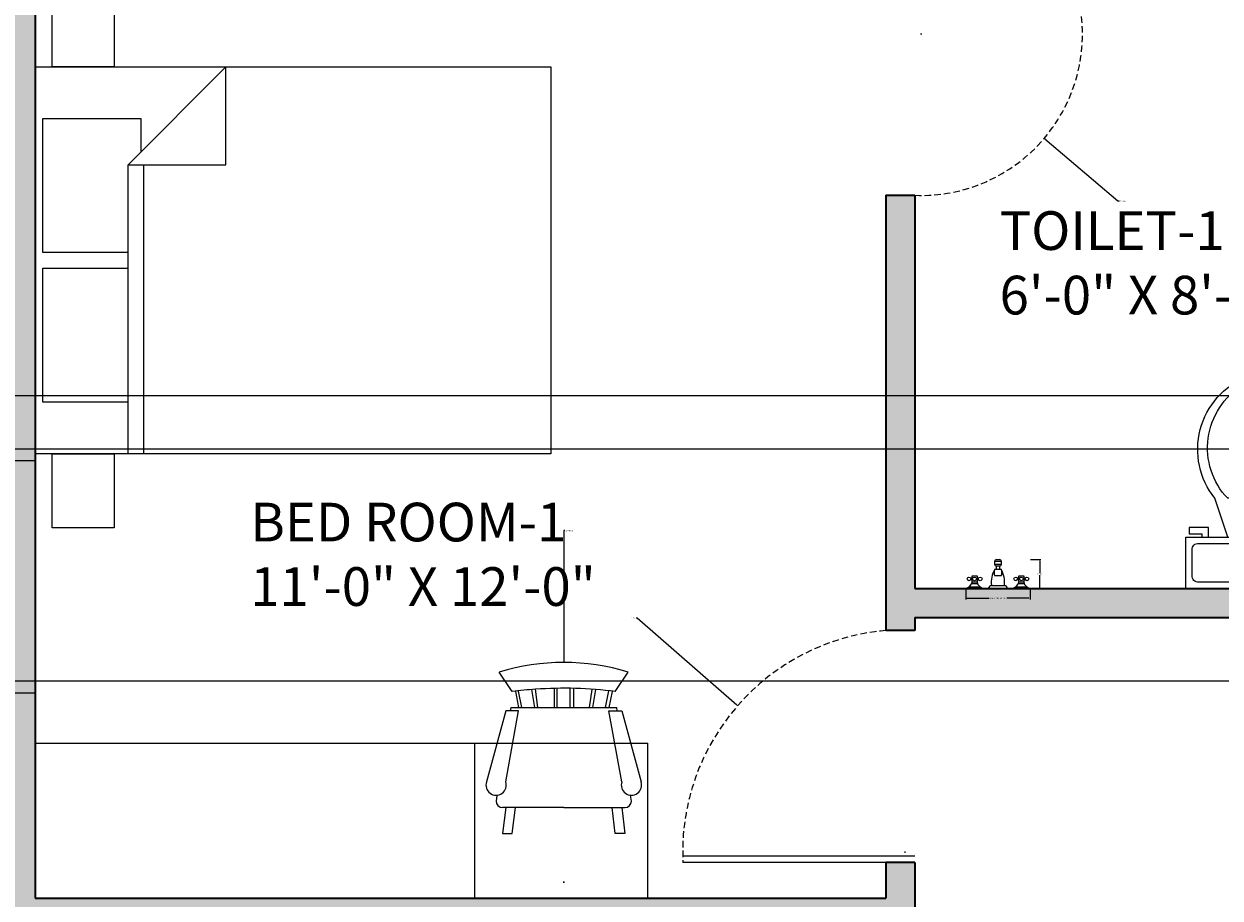
# Model space of a CAD drawing. Units: inches. Extents: x 1693 to 2974, y 2201 to 2965.
# Tile 5 of 24: x 1790 to 1976, y 2554 to 2689. Entities that reach past the tile are written whole.
import ezdxf

# ---------------------------------------------------------------- set-up
doc = ezdxf.new("R2010")
doc.units = ezdxf.units.IN
doc.header["$LTSCALE"] = 2
doc.header["$MEASUREMENT"] = 0
doc.linetypes.add('HIDDEN', pattern=[0.375, 0.25, -0.125])
for name, color, linetype, lineweight in [('A-ANNO-DIMS', 2, 'Continuous', 18), ('A-AREA-IDEN', 7, 'Continuous', 18), ('A-DOOR', 3, 'Continuous', 25), ('A-DOOR-SWNG', 3, 'HIDDEN', 13), ('A-FLOR-CASE', 32, 'Continuous', 18), ('A-FLOR-FIXT', 9, 'Continuous', 18), ('A-FURN', 8, 'Continuous', 18), ('A-GLAZ', 4, 'Continuous', 18), ('A-WALL', 7, 'Continuous', 35)]:
    doc.layers.add(name, color=color, linetype=linetype, lineweight=lineweight)
doc.layers.add('A-GLAZ-PATT', color=141, linetype='Continuous', lineweight=13, true_color=0xadddf7)
doc.layers.add('A-WALL-PATT', color=251, linetype='Continuous', lineweight=13, true_color=0x636466)
doc.styles.get("Standard").update_dxf_attribs({"font": 'arial.ttf'})
doc.dimstyles.get("Standard").update_dxf_attribs({"dimtxt": 0.18, "dimasz": 0.18, "dimexe": 0.18, "dimexo": 0.0625, "dimgap": 0.09, "dimtad": 0, "dimtih": 1, "dimtoh": 1, "dimdec": 1, "dimzin": 0, "dimdsep": 46, "dimlunit": 3, "dimtxsty": 'Standard', "dimcen": 0.09, "dimadec": 0, "dimazin": 0, "dimtfac": 1, "dimtdec": 1, "dimtofl": 0, "dimtmove": 0, "dimatfit": 3, "dimfxl": 1, "dimtolj": 1, "dimtzin": 0, "dimarcsym": 0})

# ---------------------------------------------------------------- blocks, each defined once
blk = doc.blocks.new('Chair - Rocking')
for p, q in [((-8, -4.5), (-10, -1.5)), ((8, -4.5), (10, -1.5)), ((-7.5, -4.5), (-7, -7)), ((-6.5, -7), (-7.02225, -4.43)), ((-4.5, -7), (-4.96674, -4.19951)), ((-4, -7), (-4.40532, -4.16272)), ((-1.5, -4.05012), (-1.5, -7)), ((-1, -7), (-1, -4.05012)), ((1, -7), (1, -4.04655)), ((1.5, -4.05012), (1.5, -7)), ((4, -7), (4.40187, -4.18694)), ((4.5, -7), (4.96761, -4.19437)), ((6.5, -7), (7, -4.4057)), ((7.5, -4.5), (7, -7)), ((-8.23428, -6.99939), (-8.3093, -7.47958)), ((-8.23041, -7), (8.23915, -7)), ((8.31071, -7.48854), (8.23449, -7.00073)), ((-9, -7.5), (-12, -18.49999)), ((-7, -7.5), (-9, -7.5)), ((-9, -18.49999), (-7, -7.5)), ((7, -7.5), (9, -7.5)), ((9, -18.49999), (7, -7.5)), ((9, -7.5), (12, -18.49999)), ((-10.36644, -20.64523), (-10.5, -21.49999)), ((10.5, -21.49999), (10.3575, -20.58798)), ((-9, -22.49999), (-9.5, -26.49999)), ((0, -22.49999), (-9.5, -22.49999)), ((-8, -26.49999), (-7.5, -22.49999)), ((0, -22.49999), (9.5, -22.49999)), ((8, -26.49999), (7.5, -22.49999)), ((9, -22.49999), (9.5, -26.49999)), ((-9.5, -26.49999), (-8, -26.49999)), ((9.5, -26.49999), (8, -26.49999))]:
    blk.add_line(p, q)
for centre, radius, start, end in [((0, -34.08333), 34.08333, 72.93847, 107.0615), ((0, -68.25004), 64.25, 93.92211, 97.15267), ((0, -68.25004), 64.25, 82.84733, 93.92211), ((-10.5, -18.99999), 1.58114, 161.5651, 18.43495), ((10.5, -18.99999), 1.58114, 161.5651, 18.43495), ((-9.5, -21.49999), 1, 180, 270), ((9.5, -21.49999), 1, 270, 0)]:
    blk.add_arc(centre, radius, start, end)
blk = doc.blocks.new('Bed - Queen')
for p, q in [((0, -80.00003), (0, 0)), ((0, 0), (59.99999, 0)), ((59.99999, 0), (59.99999, -80.00003)), ((7.99999, -1.2), (28.79998, -1.2)), ((7.99999, -14.4), (7.99999, -1.2)), ((28.79998, -1.2), (28.79998, -14.4)), ((31.19999, -1.2), (51.99999, -1.2)), ((31.19999, -14.4), (31.19999, -1.2)), ((51.99999, -1.2), (51.99999, -16.4)), ((0, -14.4), (44.8, -14.4)), ((59.99999, -29.6), (44.8, -14.4)), ((44.8, -14.4), (44.8, -29.6)), ((51.99999, -16.4), (46.79936, -16.4)), ((44.8, -16.8), (0, -16.8)), ((44.8, -29.6), (59.99999, -29.6)), ((59.99999, -80.00003), (0, -80.00003))]:
    blk.add_line(p, q)
blk = doc.blocks.new('Toilet - top')
for p, q in [((9.5, -6), (9.5, -2)), ((-10, -8.5), (-8, -8.5)), ((-10, -9.5), (-10, -8.5)), ((-8, -8.5), (-8, -8)), ((-7, -8), (-7, -9.5)), ((-4, -8), (-6, -14)), ((4, -8), (6, -14)), ((-7, -9.5), (-10, -9.5)), ((4, -14), (-4, -14))]:
    blk.add_line(p, q)
blk.add_lwpolyline([(10.5, -8), (10.5, 0), (-10.5, 0), (-10.5, -8)], close=True)
for points in [[(8.5, -1), (-8.5, -1)], [(-9.5, -2), (-9.5, -6)], [(-8.5, -7), (8.5, -7)]]:
    blk.add_lwpolyline(points)
for centre, radius, start, end in [((-8.62, -1.88), 0.884, 81.8699, 188.1301), ((8.62, -1.88), 0.884, 351.8699, 98.1301), ((-8.62, -6.12), 0.884, 171.8699, 278.1301), ((8.62, -6.12), 0.884, 261.8699, 8.1301), ((3.52, -21.58), 12.17, 141.4691, 247.9714), ((4.2, -21.82), 11.33, 136.3677, 238.9468), ((-3.52, -21.58), 12.17, 292.0284, 38.5307), ((-4.2, -21.82), 11.33, 301.053, 43.6321), ((0, -27.88), 4, 245.7318, 294.2682), ((0, -29), 4, 254.8605, 285.1395)]:
    blk.add_arc(centre, radius, start, end)
blk = doc.blocks.new('Faucet - Bathroom front')
for p, q in [((-0.5, 4.25), (0.5, 4.25)), ((0.5, 3.75), (-0.5, 3.75)), ((-0.5, 3), (0.5, 3)), ((0.5, 2), (-0.5, 2)), ((-0.25, 3), (-0.25, 3.5)), ((0.25, 3.5), (0.25, 3)), ((-5, 0), (-2.25, 0)), ((-4.5087, 0.25), (-2.7408, 0.25)), ((-4, 1.625), (-4.25, 1.625)), ((-4, 1.375), (-4.25, 1.375)), ((-3.1442, 0.75), (-4.0979, 0.75)), ((-3.25, 1.625), (-3, 1.625)), ((-3.25, 1.375), (-3, 1.375)), ((-1.5, 0), (1.5, 0)), ((-1, 0.5), (1, 0.5)), ((2.25, 0), (5, 0)), ((2.7413, 0.25), (4.5092, 0.25)), ((3.25, 1.625), (3, 1.625)), ((3.25, 1.375), (3, 1.375)), ((4.1058, 0.75), (3.1521, 0.75)), ((4, 1.625), (4.25, 1.625)), ((4, 1.375), (4.25, 1.375))]:
    blk.add_line(p, q)
for points in [[(-0.5, 3.75), (-0.5, 4.25)], [(-0.25, 4.5), (0.25, 4.5)], [(0.5, 4.25), (0.5, 3.75)], [(0.25, 3.5), (-0.25, 3.5)]]:
    blk.add_lwpolyline(points)
for points in [[(-4, 1), (-4, 2), (-3.25, 2), (-3.25, 1)], [(3.25, 1), (3.25, 2), (4, 2), (4, 1)]]:
    blk.add_lwpolyline(points, close=True)
for centre in [(-4.5, 1.5), (-3.625, 1.5), (-2.75, 1.5), (2.75, 1.5), (3.625, 1.5), (4.5, 1.5)]:
    blk.add_circle(centre, 0.2795)
for centre, radius, start, end in [((-0.2575, 4.2575), 0.2426, 88.22243, 181.7776), ((-0.2575, 3.7425), 0.2426, 178.2224, 271.7776), ((0.2575, 4.2575), 0.2426, 358.2224, 91.77757), ((0.2575, 3.7425), 0.2426, 268.2224, 1.777565), ((3, 1), 4.0311, 150.2551, 187.125), ((0.6413, 2.5), 1.246, 156.3417, 203.6583), ((-3, 1), 4.0311, 352.875, 29.74488), ((-0.6413, 2.5), 1.246, 336.3417, 23.65835), ((-5.375, 1.375), 1.4252, 285.2551, 344.7449), ((-1.875, 1.375), 1.4252, 195.2551, 254.7449), ((-0.7962, -0.2038), 0.7327, 106.1502, 163.8498), ((0.7962, -0.2038), 0.7327, 16.1502, 73.84979), ((1.875, 1.375), 1.4252, 285.2551, 344.7449), ((5.375, 1.375), 1.4252, 195.2551, 254.7449)]:
    blk.add_arc(centre, radius, start, end)
blk = doc.blocks.new('NIGHTSTAND')
at = {"ltscale": 2}
blk.add_lwpolyline([(11.51, 0), (0, 0), (0, 9.62), (11.51, 9.62)], close=True, dxfattribs=at)
blk = doc.blocks.new('*D45')
at = {"layer": 'A-ANNO-DIMS', "color": 0, "lineweight": -2, "ltscale": 2, "transparency": 16777216}
for p, q in [((1936.11, 2601.78), (1936.11, 2600.16)), ((1936.29, 2600.34), (1939.76, 2600.34)), ((1945.93, 2600.34), (1942.47, 2600.34)), ((1946.11, 2601.78), (1946.11, 2600.16))]:
    blk.add_line(p, q, dxfattribs=at)
at = {"layer": 'A-ANNO-DIMS', "color": 0, "ltscale": 2, "transparency": 16777216}
for points in [[(1936.29, 2600.37), (1936.29, 2600.31), (1936.11, 2600.34)], [(1945.93, 2600.37), (1945.93, 2600.31), (1946.11, 2600.34)]]:
    blk.add_solid(points, dxfattribs=at)
at = {"layer": 'Defpoints', "color": 0, "ltscale": 2, "transparency": 16777216}
for p in [(1936.11, 2601.84), (1946.11, 2601.84), (1946.11, 2600.34)]:
    blk.add_point(p, dxfattribs=at)
at = {"layer": 'A-ANNO-DIMS', "color": 0, "ltscale": 2, "transparency": 16777216, "insert": (1941.11, 2600.34), "char_height": 0.18, "attachment_point": 5}
blk.add_mtext('\\A1;TAP - FRONT 10 TYP.', dxfattribs=at)
blk = doc.blocks.new('*D46')
at = {"layer": 'A-ANNO-DIMS', "color": 0, "lineweight": -2, "ltscale": 2, "transparency": 16777216}
for p, q in [((1946.18, 2606.35), (1947.79, 2606.35)), ((1947.61, 2606.17), (1947.61, 2604.28)), ((1947.61, 2602.02), (1947.61, 2603.91)), ((1946.18, 2601.84), (1947.79, 2601.84))]:
    blk.add_line(p, q, dxfattribs=at)
at = {"layer": 'A-ANNO-DIMS', "color": 0, "ltscale": 2, "transparency": 16777216}
for points in [[(1947.58, 2606.17), (1947.64, 2606.17), (1947.61, 2606.35)], [(1947.58, 2602.02), (1947.64, 2602.02), (1947.61, 2601.84)]]:
    blk.add_solid(points, dxfattribs=at)
at = {"layer": 'Defpoints', "color": 0, "ltscale": 2, "transparency": 16777216}
for p in [(1946.11, 2606.35), (1947.61, 2606.35), (1946.11, 2601.84)]:
    blk.add_point(p, dxfattribs=at)
at = {"layer": 'A-ANNO-DIMS', "color": 0, "ltscale": 2, "transparency": 16777216, "insert": (1947.61, 2604.1), "char_height": 0.18, "attachment_point": 5}
blk.add_mtext('\\A1;5 TYP.', dxfattribs=at)
blk = doc.blocks.new('*D81')
at = {"layer": 'A-ANNO-DIMS', "color": 0, "lineweight": -2, "ltscale": 2, "transparency": 16777216}
for p, q in [((1752.34, 2553.91), (1752.34, 2964.96)), ((1752.52, 2964.78), (2332.94, 2964.78)), ((2914.06, 2964.78), (2333.64, 2964.78)), ((2914.24, 2754.97), (2914.24, 2964.96))]:
    blk.add_line(p, q, dxfattribs=at)
at = {"layer": 'A-ANNO-DIMS', "color": 0, "ltscale": 2, "transparency": 16777216}
for points in [[(1752.52, 2964.81), (1752.52, 2964.75), (1752.34, 2964.78)], [(2914.06, 2964.81), (2914.06, 2964.75), (2914.24, 2964.78)]]:
    blk.add_solid(points, dxfattribs=at)
at = {"layer": 'Defpoints', "color": 0, "ltscale": 2, "transparency": 16777216}
for p in [(2914.24, 2964.78), (2914.24, 2754.9), (1752.34, 2553.84)]:
    blk.add_point(p, dxfattribs=at)
at = {"layer": 'A-ANNO-DIMS', "color": 0, "ltscale": 2, "transparency": 16777216, "insert": (2333.29, 2964.78), "char_height": 0.18, "attachment_point": 5}
blk.add_mtext('\\A1;1162', dxfattribs=at)
blk = doc.blocks.new('*D82')
at = {"layer": 'A-ANNO-DIMS', "color": 0, "lineweight": -2, "ltscale": 2, "transparency": 16777216}
for p, q in [((2615.67, 2906.08), (1693.46, 2906.08)), ((1693.64, 2905.9), (1693.64, 2582.94)), ((1693.64, 2259.62), (1693.64, 2582.58)), ((2096.17, 2259.44), (1693.46, 2259.44))]:
    blk.add_line(p, q, dxfattribs=at)
at = {"layer": 'A-ANNO-DIMS', "color": 0, "ltscale": 2, "transparency": 16777216}
for points in [[(1693.61, 2905.9), (1693.67, 2905.9), (1693.64, 2906.08)], [(1693.61, 2259.62), (1693.67, 2259.62), (1693.64, 2259.44)]]:
    blk.add_solid(points, dxfattribs=at)
at = {"layer": 'Defpoints', "color": 0, "ltscale": 2, "transparency": 16777216}
for p in [(1693.64, 2906.08), (2615.74, 2906.08), (2096.24, 2259.44)]:
    blk.add_point(p, dxfattribs=at)
at = {"layer": 'A-ANNO-DIMS', "color": 0, "ltscale": 2, "transparency": 16777216, "insert": (1693.64, 2582.76), "char_height": 0.18, "attachment_point": 5}
blk.add_mtext('\\A1;646.6', dxfattribs=at)
blk = doc.blocks.new('*D88')
at = {"layer": 'A-ANNO-DIMS', "color": 0, "lineweight": -2, "ltscale": 2, "transparency": 16777216}
for p, q in [((2479.17, 2700.75), (1693.46, 2700.75)), ((1693.64, 2700.57), (1693.64, 2666.44)), ((1693.64, 2631.93), (1693.64, 2666.07)), ((2479.17, 2631.75), (1693.46, 2631.75))]:
    blk.add_line(p, q, dxfattribs=at)
at = {"layer": 'A-ANNO-DIMS', "color": 0, "ltscale": 2, "transparency": 16777216}
for points in [[(1693.61, 2700.57), (1693.67, 2700.57), (1693.64, 2700.75)], [(1693.61, 2631.93), (1693.67, 2631.93), (1693.64, 2631.75)]]:
    blk.add_solid(points, dxfattribs=at)
at = {"layer": 'Defpoints', "color": 0, "ltscale": 2, "transparency": 16777216}
for p in [(1693.64, 2700.75), (2479.24, 2700.75), (2479.24, 2631.75)]:
    blk.add_point(p, dxfattribs=at)
at = {"layer": 'A-ANNO-DIMS', "color": 0, "ltscale": 2, "transparency": 16777216, "insert": (1693.64, 2666.25), "char_height": 0.18, "attachment_point": 5}
blk.add_mtext('\\A1;69', dxfattribs=at)
blk = doc.blocks.new('*D98')
at = {"layer": 'A-ANNO-DIMS', "color": 0, "lineweight": -2, "ltscale": 2, "transparency": 16777216}
for p, q in [((2479.17, 2623.46), (1693.46, 2623.46)), ((1693.64, 2623.28), (1693.64, 2605.64)), ((1693.64, 2587.64), (1693.64, 2605.28)), ((2479.17, 2587.46), (1693.46, 2587.46))]:
    blk.add_line(p, q, dxfattribs=at)
at = {"layer": 'A-ANNO-DIMS', "color": 0, "ltscale": 2, "transparency": 16777216}
for points in [[(1693.61, 2623.28), (1693.67, 2623.28), (1693.64, 2623.46)], [(1693.61, 2587.64), (1693.67, 2587.64), (1693.64, 2587.46)]]:
    blk.add_solid(points, dxfattribs=at)
at = {"layer": 'Defpoints', "color": 0, "ltscale": 2, "transparency": 16777216}
for p in [(1693.64, 2623.46), (2479.24, 2623.46), (2479.24, 2587.46)]:
    blk.add_point(p, dxfattribs=at)
at = {"layer": 'A-ANNO-DIMS', "color": 0, "ltscale": 2, "transparency": 16777216, "insert": (1693.64, 2605.46), "char_height": 0.18, "attachment_point": 5}
blk.add_mtext('\\A1;36', dxfattribs=at)
blk = doc.blocks.new('*D99')
at = {"layer": 'A-ANNO-DIMS', "color": 0, "lineweight": -2, "ltscale": 2, "transparency": 16777216}
for p, q in [((2479.17, 2631.75), (1693.46, 2631.75)), ((1693.64, 2631.57), (1693.64, 2627.79)), ((1693.64, 2623.64), (1693.64, 2627.43)), ((2479.17, 2623.46), (1693.46, 2623.46))]:
    blk.add_line(p, q, dxfattribs=at)
at = {"layer": 'A-ANNO-DIMS', "color": 0, "ltscale": 2, "transparency": 16777216}
for points in [[(1693.61, 2631.57), (1693.67, 2631.57), (1693.64, 2631.75)], [(1693.61, 2623.64), (1693.67, 2623.64), (1693.64, 2623.46)]]:
    blk.add_solid(points, dxfattribs=at)
at = {"layer": 'Defpoints', "color": 0, "ltscale": 2, "transparency": 16777216}
for p in [(1693.64, 2631.75), (2479.24, 2631.75), (2479.24, 2623.46)]:
    blk.add_point(p, dxfattribs=at)
at = {"layer": 'A-ANNO-DIMS', "color": 0, "ltscale": 2, "transparency": 16777216, "insert": (1693.64, 2627.61), "char_height": 0.18, "attachment_point": 5}
blk.add_mtext('\\A1;8.295', dxfattribs=at)
blk = doc.blocks.new('*D113')
at = {"layer": 'A-ANNO-DIMS', "color": 0, "lineweight": -2, "ltscale": 2, "transparency": 16777216}
for p, q in [((1884.98, 2597.32), (1885.16, 2597.32)), ((1885.16, 2597.32), (1900.6, 2583.81)), ((1926.61, 2560.97), (1926.79, 2560.97)), ((1926.7, 2560.88), (1926.7, 2561.06))]:
    blk.add_line(p, q, dxfattribs=at)
at = {"layer": 'A-ANNO-DIMS', "color": 0, "ltscale": 2, "transparency": 16777216}
blk.add_solid([(1900.62, 2583.83), (1900.58, 2583.79), (1900.73, 2583.69)], dxfattribs=at)
at = {"layer": 'Defpoints', "color": 0, "ltscale": 2, "transparency": 16777216}
for p in [(1900.73, 2583.69), (1926.7, 2560.97)]:
    blk.add_point(p, dxfattribs=at)
at = {"layer": 'A-ANNO-DIMS', "color": 0, "ltscale": 2, "transparency": 16777216, "insert": (1884.57, 2597.32), "char_height": 0.18, "attachment_point": 5}
blk.add_mtext('\\A1;R34.5', dxfattribs=at)
blk = doc.blocks.new('*D125')
at = {"layer": 'A-ANNO-DIMS', "color": 0, "lineweight": -2, "ltscale": 2, "transparency": 16777216}
for p, q in [((1929.1, 2687.87), (1929.28, 2687.87)), ((1929.19, 2687.78), (1929.19, 2687.96)), ((1959.72, 2661.92), (1948.41, 2671.53)), ((1959.9, 2661.92), (1959.72, 2661.92))]:
    blk.add_line(p, q, dxfattribs=at)
at = {"layer": 'A-ANNO-DIMS', "color": 0, "ltscale": 2, "transparency": 16777216}
blk.add_solid([(1948.43, 2671.56), (1948.39, 2671.51), (1948.27, 2671.65)], dxfattribs=at)
at = {"layer": 'Defpoints', "color": 0, "ltscale": 2, "transparency": 16777216}
for p in [(1929.19, 2687.87), (1948.27, 2671.65)]:
    blk.add_point(p, dxfattribs=at)
at = {"layer": 'A-ANNO-DIMS', "color": 0, "ltscale": 2, "transparency": 16777216, "insert": (1960.45, 2661.92), "char_height": 0.18, "attachment_point": 5}
blk.add_mtext('\\A1;R25.044', dxfattribs=at)
blk = doc.blocks.new('*D130')
at = {"layer": 'A-ANNO-DIMS', "color": 0, "lineweight": -2, "ltscale": 2, "transparency": 16777216}
for p, q in [((1873.93, 2610.83), (1873.75, 2610.83)), ((1873.75, 2610.83), (1873.75, 2590.56)), ((1873.66, 2556.3), (1873.84, 2556.3)), ((1873.75, 2556.21), (1873.75, 2556.39))]:
    blk.add_line(p, q, dxfattribs=at)
at = {"layer": 'A-ANNO-DIMS', "color": 0, "ltscale": 2, "transparency": 16777216}
blk.add_solid([(1873.72, 2590.56), (1873.78, 2590.56), (1873.75, 2590.38)], dxfattribs=at)
at = {"layer": 'Defpoints', "color": 0, "ltscale": 2, "transparency": 16777216}
for p in [(1873.75, 2590.38), (1873.75, 2556.3)]:
    blk.add_point(p, dxfattribs=at)
at = {"layer": 'A-ANNO-DIMS', "color": 0, "ltscale": 2, "transparency": 16777216, "insert": (1874.6, 2610.83), "char_height": 0.18, "attachment_point": 5}
blk.add_mtext('\\A1;2X R34.08', dxfattribs=at)

msp = doc.modelspace()

# ---------------------------------------------------------------- hatches: boundary and pattern name
at = {"layer": 'A-GLAZ-PATT', "ltscale": 2}
h = msp.add_hatch(color=256, dxfattribs=at)
h.dxf.hatch_style = 1
h.paths.add_polyline_path([(2656.9702, 2338.2547), (2632.9702, 2338.2547), (2632.9702, 2339.2547), (2608.9702, 2339.2547), (2608.9702, 2334.7547), (2656.9702, 2334.7547)])
h.paths.add_polyline_path([(2656.9702, 2343.7547), (2608.9702, 2343.7547), (2608.9702, 2340.2547), (2632.9702, 2340.2547), (2632.9702, 2339.2547), (2656.9702, 2339.2547)])
h.paths.add_polyline_path([(2775.7544, 2338.2547), (2751.7544, 2338.2547), (2751.7544, 2334.7547), (2775.7544, 2334.7547)])
h.paths.add_polyline_path([(2775.7544, 2343.7547), (2751.7544, 2343.7547), (2751.7544, 2340.2547), (2775.7544, 2340.2547)])
h.paths.add_polyline_path([(2897.7363, 2568.7999), (2893.2363, 2568.7999), (2893.2363, 2520.7999), (2896.7363, 2520.7999), (2896.7363, 2544.7999), (2897.7363, 2544.7999)])
h.paths.add_polyline_path([(2902.2363, 2568.7999), (2898.7363, 2568.7999), (2898.7363, 2544.7999), (2897.7363, 2544.7999), (2897.7363, 2520.7999), (2902.2363, 2520.7999)])
h.paths.add_polyline_path([(2902.2363, 2637.7547), (2898.7363, 2637.7547), (2898.7363, 2613.7547), (2902.2363, 2613.7547)])
h.paths.add_polyline_path([(2896.7363, 2637.7547), (2893.2363, 2637.7547), (2893.2363, 2613.7547), (2896.7363, 2613.7547)])
h.paths.add_polyline_path([(2902.2363, 2748.903), (2899.0477, 2748.903), (2899.0477, 2724.903), (2898.0477, 2724.903), (2898.0477, 2700.903), (2902.2363, 2700.903)])
h.paths.add_polyline_path([(2898.0477, 2748.903), (2893.2363, 2748.903), (2893.2363, 2700.903), (2897.0477, 2700.903), (2897.0477, 2724.903), (2898.0477, 2724.903)])
h.paths.add_polyline_path([(2851.2363, 2846.2547), (2803.2363, 2846.2547), (2803.2363, 2842.7547), (2827.2363, 2842.7547), (2827.2363, 2841.7547), (2851.2363, 2841.7547)])
h.paths.add_polyline_path([(2851.2363, 2840.7547), (2827.2363, 2840.7547), (2827.2363, 2841.7547), (2803.2363, 2841.7547), (2803.2363, 2837.2547), (2851.2363, 2837.2547)])
h.paths.add_polyline_path([(2578.2363, 2846.2547), (2530.2363, 2846.2547), (2530.2363, 2842.7547), (2554.2363, 2842.7547), (2554.2363, 2841.7547), (2578.2363, 2841.7547)])
h.paths.add_polyline_path([(2578.2363, 2840.7547), (2554.2363, 2840.7547), (2554.2363, 2841.7547), (2530.2363, 2841.7547), (2530.2363, 2837.2547), (2578.2363, 2837.2547)])
h.paths.add_polyline_path([(2732.7363, 2812.7547), (2705.1363, 2812.7547), (2705.1363, 2811.7547), (2676.3363, 2811.7547), (2676.3363, 2812.7547), (2648.7363, 2812.7547), (2648.7363, 2808.2547), (2732.7363, 2808.2547)])
h.paths.add_polyline_path([(2732.7363, 2817.2547), (2648.7363, 2817.2547), (2648.7363, 2813.7547), (2676.3363, 2813.7547), (2676.3363, 2812.7547), (2705.1363, 2812.7547), (2705.1363, 2813.7547), (2732.7363, 2813.7547)])
h.paths.add_polyline_path([(2488.2363, 2695.8203), (2484.7878, 2695.8203), (2484.7878, 2671.8203), (2488.2363, 2671.8203)])
h.paths.add_polyline_path([(2482.7878, 2695.8203), (2479.2363, 2695.8203), (2479.2363, 2671.8203), (2482.7878, 2671.8203)])
h.paths.add_polyline_path([(2488.2363, 2572.4371), (2484.7363, 2572.4371), (2484.7363, 2541.4371), (2483.7363, 2541.4371), (2483.7363, 2512.4371), (2488.2363, 2512.4371)])
h.paths.add_polyline_path([(2482.7363, 2541.4371), (2483.7363, 2541.4371), (2483.7363, 2572.4371), (2479.2363, 2572.4371), (2479.2363, 2512.4371), (2482.7363, 2512.4371)])
h.paths.add_polyline_path([(2248.9863, 2706.8449), (2190.9863, 2706.8449), (2190.9863, 2703.3449), (2219.9863, 2703.3449), (2219.9863, 2702.3449), (2248.9863, 2702.3449)])
h.paths.add_polyline_path([(2248.9863, 2701.3449), (2219.9863, 2701.3449), (2219.9863, 2702.3449), (2190.9863, 2702.3449), (2190.9863, 2697.8449), (2248.9863, 2697.8449)])
h.paths.add_polyline_path([(2151.9207, 2293.3449), (2127.9207, 2293.3449), (2127.9207, 2289.8449), (2151.9207, 2289.8449)])
h.paths.add_polyline_path([(2151.9207, 2298.8449), (2127.9207, 2298.8449), (2127.9207, 2295.3449), (2151.9207, 2295.3449)])
h.paths.add_polyline_path([(2084.023, 2293.3449), (2066.023, 2293.3449), (2066.023, 2294.3449), (2048.023, 2294.3449), (2048.023, 2289.8449), (2084.023, 2289.8449)])
h.paths.add_polyline_path([(2084.023, 2298.8449), (2048.023, 2298.8449), (2048.023, 2295.3449), (2066.023, 2295.3449), (2066.023, 2294.3449), (2084.023, 2294.3449)])
h.paths.add_polyline_path([(1966.0781, 2293.3449), (1948.0781, 2293.3449), (1948.0781, 2294.3449), (1930.0781, 2294.3449), (1930.0781, 2289.8449), (1966.0781, 2289.8449)])
h.paths.add_polyline_path([(1966.0781, 2298.8449), (1930.0781, 2298.8449), (1930.0781, 2295.3449), (1948.0781, 2295.3449), (1948.0781, 2294.3449), (1966.0781, 2294.3449)])
h.paths.add_polyline_path([(1787.2363, 2403.1922), (1782.7363, 2403.1922), (1782.7363, 2355.1922), (1786.2363, 2355.1922), (1786.2363, 2379.1922), (1787.2363, 2379.1922)])
h.paths.add_polyline_path([(1791.7363, 2403.1922), (1788.2363, 2403.1922), (1788.2363, 2379.1922), (1787.2363, 2379.1922), (1787.2363, 2355.1922), (1791.7363, 2355.1922)])
h.paths.add_polyline_path([(1786.2363, 2477.5455), (1782.7363, 2477.5455), (1782.7363, 2453.5455), (1786.2363, 2453.5455)])
h.paths.add_polyline_path([(1791.7363, 2477.5455), (1788.2363, 2477.5455), (1788.2363, 2453.5455), (1791.7363, 2453.5455)])
h.paths.add_polyline_path([(1786.2363, 2621.6433), (1782.7363, 2621.6433), (1782.7363, 2585.6433), (1786.2363, 2585.6433)])
h.paths.add_polyline_path([(1791.7363, 2621.6433), (1788.2363, 2621.6433), (1788.2363, 2585.6433), (1791.7363, 2585.6433)])
h.paths.add_polyline_path([(1908.1286, 2706.8449), (1860.1286, 2706.8449), (1860.1286, 2703.3449), (1884.1286, 2703.3449), (1884.1286, 2702.3449), (1908.1286, 2702.3449)])
h.paths.add_polyline_path([(1908.1286, 2701.3449), (1884.1286, 2701.3449), (1884.1286, 2702.3449), (1860.1286, 2702.3449), (1860.1286, 2697.8449), (1908.1286, 2697.8449)])
h.paths.add_polyline_path([(1973.9863, 2706.8449), (1949.9863, 2706.8449), (1949.9863, 2703.3449), (1973.9863, 2703.3449)])
h.paths.add_polyline_path([(1973.9863, 2701.3449), (1949.9863, 2701.3449), (1949.9863, 2697.8449), (1973.9863, 2697.8449)])
h.paths.add_polyline_path([(2112.7363, 2690.3449), (2028.7363, 2690.3449), (2028.7363, 2686.8449), (2056.3363, 2686.8449), (2056.3363, 2685.8449), (2085.1363, 2685.8449), (2085.1363, 2686.8449), (2112.7363, 2686.8449)])
h.paths.add_polyline_path([(2112.7363, 2685.8449), (2085.1363, 2685.8449), (2085.1363, 2684.8449), (2056.3363, 2684.8449), (2056.3363, 2685.8449), (2028.7363, 2685.8449), (2028.7363, 2681.3449), (2112.7363, 2681.3449)])
h.paths.add_polyline_path([(2422.7363, 2640.7547), (2350.7363, 2640.7547), (2350.7363, 2637.2547), (2386.7363, 2637.2547), (2386.7363, 2636.2547), (2422.7363, 2636.2547)])
h.paths.add_polyline_path([(2422.7363, 2635.2547), (2386.7363, 2635.2547), (2386.7363, 2636.2547), (2350.7363, 2636.2547), (2350.7363, 2631.7547), (2422.7363, 2631.7547)])
at = {"layer": 'A-WALL-PATT', "ltscale": 2}
h = msp.add_hatch(color=256, dxfattribs=at)
h.dxf.hatch_style = 1
h.paths.add_polyline_path([(1928.2363, 2733.2161), (1930.9384, 2733.2161), (1930.9384, 2737.2161), (1923.7363, 2737.2161), (1923.7363, 2706.8449), (1908.1286, 2706.8449), (1908.1286, 2697.8449), (1923.7363, 2697.8449), (1923.7363, 2692.8449), (1928.2363, 2692.8449), (1928.2363, 2697.8449), (1949.9863, 2697.8449), (1949.9863, 2706.8449), (1928.2363, 2706.8449)])
h.paths.add_polyline_path([(2004.7363, 2737.2161), (1995.7363, 2737.2161), (1995.7363, 2706.8449), (1985.6374, 2706.8449), (1973.9863, 2706.8449), (1973.9863, 2697.8449), (2000.2363, 2697.8449), (2000.2363, 2686.5348), (2000.3613, 2686.5348), (2000.3613, 2667.0432), (2000.2363, 2601.8449), (1928.2363, 2601.8449), (1928.2363, 2662.8449), (1923.7363, 2662.8449), (1923.7363, 2595.3449), (1928.2363, 2595.3449), (1928.2363, 2597.3449), (2004.7363, 2597.3449), (2004.7363, 2681.3449), (2012.7814, 2681.3449), (2028.7363, 2681.3449), (2028.7363, 2690.3449), (2004.7363, 2690.3449)])
h.paths.add_polyline_path([(2190.9863, 2706.8449), (2184.9863, 2706.8449), (2145.7363, 2706.8449), (2145.7363, 2765.3449), (2145.7363, 2774.5394), (2136.7363, 2774.5394), (2136.7363, 2756.3449), (2136.7363, 2690.3449), (2112.7363, 2690.3449), (2112.7363, 2681.3449), (2136.7363, 2681.3449), (2136.7363, 2597.3449), (2141.2363, 2597.3449), (2141.2363, 2697.8449), (2190.9863, 2697.8449)])
h.paths.add_polyline_path([(1860.1286, 2706.8449), (1782.7363, 2706.8449), (1782.7363, 2621.6433), (1791.7363, 2621.6433), (1791.7363, 2697.8449), (1860.1286, 2697.8449)])
h.paths.add_polyline_path([(1791.7363, 2585.6433), (1782.7363, 2585.6433), (1782.7363, 2562.8449), (1782.7363, 2553.8449), (1752.3363, 2553.8449), (1752.3363, 2544.2586), (1756.3363, 2544.2586), (1756.3363, 2549.3449), (1782.7363, 2549.3449), (1782.7363, 2489.2404), (1782.7363, 2477.5455), (1791.7363, 2477.5455), (1791.7363, 2493.5991), (1791.6113, 2493.5991), (1791.6113, 2513.0907), (1791.6824, 2533.7198, -0.94742783), (1791.7363, 2534.7168), (1791.7363, 2549.3449), (1863.7363, 2549.3449), (1863.7363, 2513.3449), (1866.7363, 2513.3449), (1866.7363, 2549.3449), (1924.7363, 2549.3449), (1924.7363, 2447.3449), (1924.7363, 2442.8449), (1933.7363, 2442.8449), (1933.7363, 2447.3449), (1928.2363, 2447.3449), (1928.2363, 2559.3449), (1923.7363, 2559.3449), (1923.7363, 2553.8449), (1791.7363, 2553.8449), (1791.7363, 2562.8449)])
h.paths.add_polyline_path([(1791.7363, 2442.8449), (1866.7363, 2442.8449), (1866.7363, 2447.3449), (1866.7363, 2483.3449), (1863.7363, 2483.3449), (1863.7363, 2447.3449), (1791.7363, 2447.3449), (1791.7363, 2453.5455), (1782.7363, 2453.5455), (1782.7363, 2447.3449), (1756.3363, 2447.3449), (1756.3363, 2455.7126), (1752.3363, 2455.7126), (1752.3363, 2442.8449), (1782.7363, 2442.8449), (1782.7363, 2403.1922), (1791.7363, 2403.1922)])
h.paths.add_polyline_path([(1930.0781, 2298.8449), (1791.7363, 2298.8449), (1791.7363, 2355.1922), (1782.7363, 2355.1922), (1782.7363, 2289.8449), (1930.0781, 2289.8449)])
h.paths.add_polyline_path([(2624.7363, 2883.2547), (2624.7363, 2902.6165), (2624.7363, 2906.0761), (2615.7363, 2906.0761), (2615.7363, 2892.2547), (2615.7363, 2846.2547), (2578.2363, 2846.2547), (2578.2363, 2837.2547), (2620.2363, 2837.2547), (2620.2363, 2743.2547), (2624.7363, 2743.2547), (2624.7363, 2808.2547), (2648.7363, 2808.2547), (2648.7363, 2817.2547), (2624.7363, 2817.2547)])
h.paths.add_polyline_path([(2530.2363, 2846.2547), (2479.2363, 2846.2547), (2479.2363, 2695.8203), (2488.2363, 2695.8203), (2488.2363, 2700.7547), (2567.2363, 2700.7547), (2567.2363, 2705.2547), (2488.2363, 2705.2547), (2488.2363, 2837.2547), (2530.2363, 2837.2547)])
h.paths.add_polyline_path([(2488.2363, 2487.7547), (2630.2363, 2487.7547, -0.00990191), (2630.2363, 2489.0322), (2630.2363, 2492.2547), (2488.2363, 2492.2547), (2488.2363, 2512.4371), (2479.2363, 2512.4371), (2479.2363, 2334.7547), (2608.9702, 2334.7547), (2608.9702, 2343.7547), (2488.2363, 2343.7547)])
h.paths.add_polyline_path([(2751.7544, 2343.7547), (2672.7363, 2343.7547), (2672.7363, 2409.7547), (2674.7363, 2409.7547), (2674.7363, 2413.7547), (2672.7363, 2413.7547), (2672.7363, 2487.7547), (2732.7363, 2487.7547), (2732.7363, 2413.7547), (2704.7363, 2413.7547), (2704.7363, 2409.7547), (2784.7363, 2409.7547), (2784.7363, 2343.7547), (2775.7544, 2343.7547), (2775.7544, 2334.7547), (2902.2363, 2334.7547), (2902.2363, 2520.7999), (2893.2363, 2520.7999), (2893.2363, 2413.7547), (2856.0145, 2413.7547), (2856.0145, 2409.7547), (2893.2363, 2409.7547), (2893.2363, 2343.7547), (2789.2363, 2343.7547), (2789.2363, 2409.7547), (2819.2363, 2409.7547), (2826.0145, 2409.7547), (2826.0145, 2413.7547), (2789.2363, 2413.7547), (2789.2363, 2492.2547), (2784.7363, 2492.2547), (2784.7363, 2413.7547), (2736.7363, 2413.7547), (2736.7363, 2492.2547), (2672.7363, 2492.2547), (2666.2363, 2492.2547), (2666.2363, 2487.7547), (2668.2363, 2487.7547), (2668.2363, 2343.7547), (2656.9702, 2343.7547), (2656.9702, 2334.7547), (2662.9702, 2334.7547), (2751.7544, 2334.7547)])
h.paths.add_polyline_path([(2902.2363, 2613.7547), (2893.2363, 2613.7547), (2893.2363, 2589.7547), (2785.2363, 2589.7547), (2785.2363, 2661.7547), (2790.2363, 2661.7547), (2790.2363, 2665.2547), (2761.2363, 2665.2547), (2761.2363, 2667.2547), (2756.7363, 2667.2547), (2756.7363, 2661.7547), (2781.2363, 2661.7547), (2781.2363, 2585.7547), (2893.2363, 2585.7547), (2893.2363, 2568.7999), (2902.2363, 2568.7999)])
h.paths.add_polyline_path([(2488.2363, 2671.8203), (2479.2363, 2671.8203), (2479.2363, 2645.2547), (2479.2363, 2623.4598), (2488.2363, 2623.4598), (2488.2363, 2636.2547), (2624.7363, 2636.2547), (2624.7363, 2640.7547), (2603.7363, 2640.7547), (2603.7363, 2700.7547), (2624.7363, 2700.7547), (2624.7363, 2707.2547), (2620.2363, 2707.2547), (2620.2363, 2705.2547), (2597.2363, 2705.2547), (2597.2363, 2700.7547), (2599.2363, 2700.7547), (2599.2363, 2640.7547), (2488.2363, 2640.7547)])
h.paths.add_polyline_path([(2761.2363, 2837.2547), (2803.2363, 2837.2547), (2803.2363, 2846.2547), (2797.2363, 2846.2547), (2765.7363, 2846.2547), (2756.7363, 2846.2547), (2756.7363, 2817.2547), (2732.7363, 2817.2547), (2732.7363, 2808.2547), (2756.7363, 2808.2547), (2756.7363, 2703.2547), (2761.2363, 2703.2547)])
h.paths.add_polyline_path([(2739.7489, 2433.1234), (2786.9181, 2433.1234), (2786.9181, 2455.5122), (2739.7489, 2455.5122)], flags=25)

# ---------------------------------------------------------------- linework, layer by layer
at = {"layer": 'A-DOOR', "ltscale": 2}
for p, q in [((1928.2363, 2560.3449), (1892.2363, 2560.3449)), ((1928.2363, 2559.3449), (1892.2363, 2559.3449))]:
    msp.add_line(p, q, dxfattribs=at)
at = {"layer": 'A-DOOR-SWNG', "ltscale": 2}
for centre, radius, start, end in [((1929.1915, 2687.8705), 25.0438, 267.814245, 11.456682), ((1926.6957, 2560.9742), 34.4979, 94.921104, 182.707046)]:
    msp.add_arc(centre, radius, start, end, dxfattribs=at)
at = {"layer": 'A-FLOR-CASE'}
msp.add_line((1791.7363, 2577.8449), (1886.7942, 2577.8449), dxfattribs=at)
at = {"layer": 'A-FLOR-CASE', "ltscale": 2}
for p, q in [((1859.9709, 2553.8449), (1859.9709, 2577.8449)), ((1886.7942, 2553.8449), (1886.7942, 2577.8449))]:
    msp.add_line(p, q, dxfattribs=at)
at = {"layer": 'A-GLAZ', "ltscale": 2}
for p, q in [((1791.7363, 2621.6433), (1782.7363, 2621.6433)), ((1791.7363, 2585.6433), (1782.7363, 2585.6433))]:
    msp.add_line(p, q, dxfattribs=at)
at = {"layer": 'A-WALL'}
for p, q in [((1791.7363, 2697.8449), (1791.7363, 2562.8449)), ((1923.7363, 2662.8449), (1928.2363, 2662.8449)), ((1923.7363, 2662.8449), (1923.7363, 2595.3449)), ((1928.2363, 2662.8449), (1928.2363, 2601.8449)), ((1928.2363, 2601.8449), (2000.2363, 2601.8449)), ((1928.2363, 2597.3449), (2004.7363, 2597.3449)), ((1928.2363, 2597.3449), (1928.2363, 2595.3449)), ((1928.2363, 2595.3449), (1923.7363, 2595.3449)), ((1791.7363, 2562.8449), (1791.7363, 2553.8449)), ((1928.2363, 2559.3449), (1923.7363, 2559.3449)), ((1923.7363, 2559.3449), (1923.7363, 2553.8449)), ((1928.2363, 2559.3449), (1928.2363, 2447.3449)), ((1791.7363, 2553.8449), (1923.7363, 2553.8449))]:
    msp.add_line(p, q, dxfattribs=at)

# ---------------------------------------------------------------- block references
at = {"layer": 'A-FLOR-FIXT', "ltscale": 2, "xscale": -1, "rotation": 180}
msp.add_blockref('Toilet - top', (1980.7563, 2601.8449), dxfattribs=at)
at = {"layer": 'A-FLOR-FIXT', "ltscale": 2}
msp.add_blockref('Faucet - Bathroom front', (1941.1129, 2601.8449), dxfattribs=at)
at = {"layer": 'A-FURN'}
for p, rotation in [((1794.3504, 2694.2704), 270.0000000000054), ((1794.3504, 2622.7606), 270.0000000000035)]:
    msp.add_blockref('NIGHTSTAND', p, dxfattribs=dict(at, rotation=rotation))
at = {"layer": 'A-FURN', "ltscale": 2, "rotation": 89.99999999999999}
msp.add_blockref('Bed - Queen', (1791.7363, 2622.7605), dxfattribs=at)
at = {"layer": 'A-FURN', "ltscale": 2}
msp.add_blockref('Chair - Rocking', (1873.7457, 2590.3848), dxfattribs=at)

# ---------------------------------------------------------------- texts
at = {"layer": 'A-AREA-IDEN', "ltscale": 2, "char_height": 6, "attachment_point": 1}
for s, insert in [('TOILET-1\\P6\'-0" X 8\'-0"', (1941.3688, 2660.3674)), ('BED ROOM-1\\P11\'-0" X 12\'-0"', (1825.0984, 2615.162))]:
    msp.add_mtext_dynamic_manual_height_columns(s, width=108.452746, gutter_width=1, heights=[0], dxfattribs=dict(at, insert=insert))

# ---------------------------------------------------------------- dimensions: what is measured, and where the dimension line sits
at = {"layer": 'A-ANNO-DIMS', "ltscale": 2}
dim = msp.add_linear_dim(base=(2914.2363, 2964.7761), p1=(1752.3363, 2553.8449), p2=(2914.2363, 2754.903), dimstyle='Standard', override={"dimdec": 0, "dimlfac": 1, "dimrnd": 0, "dimzin": 0, "dimdsep": 46, "dimlunit": 2}, dxfattribs=at)
dim.commit()
dim.dimension.update_dxf_attribs({"geometry": '*D81', "text_midpoint": (2333.2863, 2964.7761)})
for base, p1, p2, override, picture, middle in [((1693.6363, 2906.0761), (2096.2363, 2259.4449), (2615.7363, 2906.0761), {"dimdec": 1, "dimlfac": 1, "dimrnd": 0, "dimzin": 0, "dimdsep": 46, "dimlunit": 2}, '*D82', (1693.6363, 2582.7605)), ((1693.6363, 2700.7547), (2479.2363, 2631.7547), (2479.2363, 2700.7547), {"dimdec": 0, "dimlfac": 1, "dimrnd": 0, "dimzin": 0, "dimdsep": 46, "dimlunit": 2}, '*D88', (1693.6363, 2666.2547)), ((1693.6363, 2631.7547), (2479.2363, 2623.4598), (2479.2363, 2631.7547), {"dimdec": 3, "dimlfac": 1, "dimrnd": 0, "dimzin": 0, "dimdsep": 46, "dimlunit": 2}, '*D99', (1693.6363, 2627.6073)), ((1693.6363, 2623.4598), (2479.2363, 2587.4598), (2479.2363, 2623.4598), {"dimdec": 0, "dimlfac": 1, "dimrnd": 0, "dimzin": 0, "dimdsep": 46, "dimlunit": 2}, '*D98', (1693.6363, 2605.4598))]:
    dim = msp.add_linear_dim(base=base, p1=p1, p2=p2, angle=90, dimstyle='Standard', override=override, dxfattribs=at)
    dim.commit()
    dim.dimension.update_dxf_attribs({"geometry": picture, "text_midpoint": middle})
for center, mpoint, override, picture, middle in [((1929.1915, 2687.8705), (1948.2732, 2671.6508), {"dimdec": 3, "dimlfac": 1, "dimrnd": 0, "dimzin": 0, "dimdsep": 46, "dimlunit": 2}, '*D125', (1960.4517, 2661.919)), ((1926.6957, 2560.9742), (1900.7331, 2583.6909), {"dimdec": 1, "dimlfac": 1, "dimrnd": 0, "dimzin": 0, "dimdsep": 46, "dimlunit": 2}, '*D113', (1884.565, 2597.3209))]:
    dim = msp.add_radius_dim(center=center, mpoint=mpoint, dimstyle='Standard', override=override, dxfattribs=at)
    dim.commit()
    dim.dimension.update_dxf_attribs({"geometry": picture, "text_midpoint": middle, "dimtype": 164})
dim = msp.add_radius_dim(center=(1873.7457, 2556.3015), mpoint=(1873.746, 2590.3848), text='2X <>', dimstyle='Standard', override={"dimdec": 2, "dimlfac": 1, "dimrnd": 0, "dimzin": 0, "dimdsep": 46, "dimlunit": 2}, dxfattribs=at)
dim.commit()
dim.dimension.update_dxf_attribs({"geometry": '*D130', "text_midpoint": (1874.6011, 2610.8348), "dimtype": 164})
dim = msp.add_linear_dim(base=(1947.6129, 2606.3469), p1=(1946.1129, 2601.8449), p2=(1946.1129, 2606.3469), angle=90, text='<> TYP.', dimstyle='Standard', override={"dimdec": 0, "dimlfac": 1, "dimrnd": 0, "dimzin": 0, "dimdsep": 46, "dimlunit": 2}, dxfattribs=at)
dim.commit()
dim.dimension.update_dxf_attribs({"geometry": '*D46', "text_midpoint": (1947.6129, 2604.0959)})
dim = msp.add_linear_dim(base=(1946.1129, 2600.3449), p1=(1936.1129, 2601.8449), p2=(1946.1129, 2601.8449), text='TAP - FRONT <> TYP.', dimstyle='Standard', override={"dimdec": 0, "dimlfac": 1, "dimrnd": 0, "dimzin": 0, "dimdsep": 46, "dimlunit": 2}, dxfattribs=at)
dim.commit()
dim.dimension.update_dxf_attribs({"geometry": '*D45', "text_midpoint": (1941.1129, 2600.3449)})

doc.saveas('drawing.dxf')
